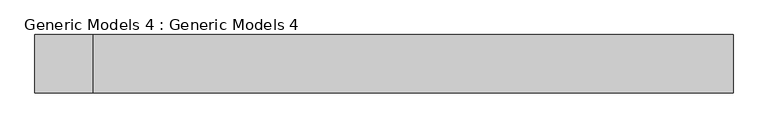
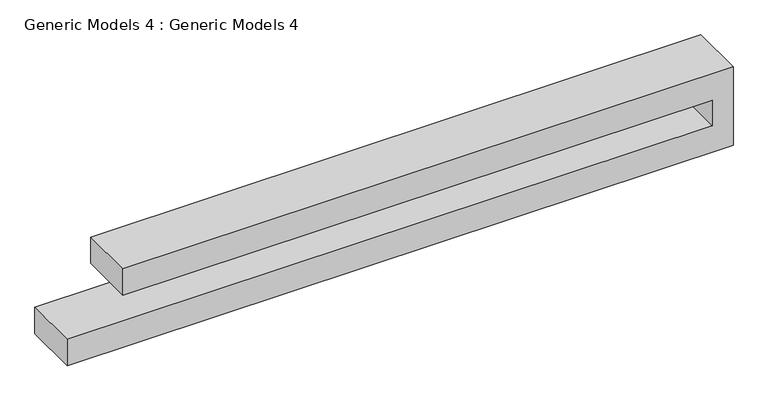
"""IFC4 building model written with IfcOpenShell, lengths in millimetres: proxy geometry, Generic Models 4 : Generic Models 4."""

from ifc_helpers import new_model, si_unit, frame, origin, place, context, project, spatial, polyline, outline, extrude, source, transform, mapped, element, save


def generic_models_4_generic_models_4_8dd9e423(model_context):
    return source(origin(), model_context, "Body", "SweptSolid", [
        extrude(outline(polyline([(7010.4, -2408.3482439), (7010.4, -9088.5482439), (6705.6, -9088.5482439), (6705.6, -2636.9482439), (6408.3761011, -2636.9482439), (6408.3761011, -9698.1482439), (6103.5761011, -9698.1482439), (6103.5761011, -2408.3482439), (7010.4, -2408.3482439)])), frame((0.0, -6332.1827462, 0.0), z_axis=(0.0, 1.0, 0.0), x_axis=(0.0, 0.0, 1.0)), (0.0, 0.0, 1.0), 609.6),
    ])


if __name__ == "__main__":
    model = new_model("IFC4")
    model_context = context("Model", 3, world=origin())
    ifc_project = project(units=[si_unit("LENGTHUNIT", "METRE", prefix="MILLI")], contexts=[model_context])
    site = spatial("IfcSite", under=ifc_project)
    building = spatial("IfcBuilding", under=site)
    placement = place(None, origin())
    generic_models_4_generic_models_4_shape = generic_models_4_generic_models_4_8dd9e423(model_context)
    element("IfcBuildingElementProxy", 1, Name="Generic Models 4 : Generic Models 4", ObjectType="Generic Models 4 : Generic Models 4", at=placement, inside=building, context=model_context, shape_type="MappedRepresentation", body=[
        mapped(generic_models_4_generic_models_4_shape, transform((0.0, 0.0, 0.0), x_axis=(1.0, 0.0, 0.0), y_axis=(0.0, 1.0, 0.0), z_axis=(0.0, 0.0, 1.0))),
    ])
    save(model, "model.ifc")
